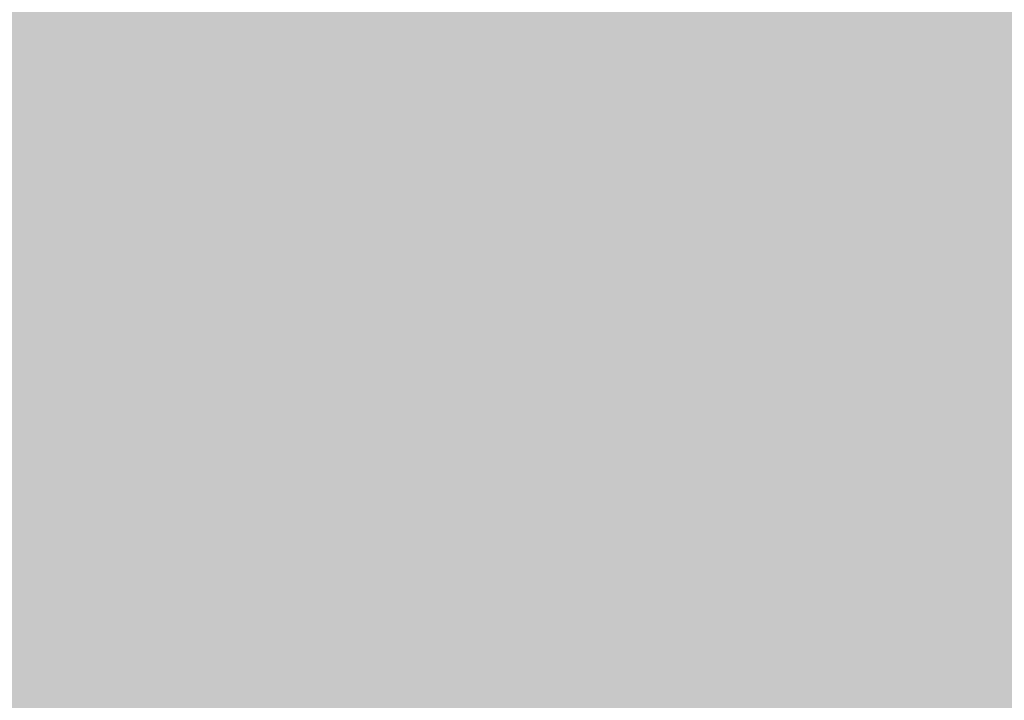
# Model space of a CAD drawing. Units: feet. Extents: x 3168 to 4724, y 827 to 1477.
# Tile 238 of 256: x 3382.8822 to 3383.8327, y 1098.344 to 1099.0007. Entities that reach past the tile are written whole.
import ezdxf

# ---------------------------------------------------------------- set-up
doc = ezdxf.new("R2010")
doc.units = ezdxf.units.FT
doc.layers.add('A-ELEV', color=7, linetype='Continuous', lineweight=35)
doc.layers.add('A-ELEV-PATT', color=8, linetype='Continuous', lineweight=13)

msp = doc.modelspace()

# ---------------------------------------------------------------- hatches: boundary and pattern name
at = {"layer": 'A-ELEV-PATT'}
h = msp.add_hatch(color=256, dxfattribs=at)
h.dxf.hatch_style = 1
edge = h.paths.add_edge_path()
edge.add_ellipse((3552.90576, 979.22014), major_axis=(36.74492, 0), ratio=0.48484848, start_angle=0, end_angle=360)
edge = h.paths.add_edge_path()
edge.add_ellipse((3559.89164, 929.25228), major_axis=(36.74492, 0), ratio=0.48484848, start_angle=0, end_angle=360)
edge = h.paths.add_edge_path()
edge.add_line((3299.31681, 1198.60608), (3479.91671, 1198.60608))
edge.add_line((3479.91671, 1198.60608), (3479.91671, 1209.86857))
edge.add_spline(control_points=[(3479.91671, 1209.86857), (3464.30116, 1209.86857), (3448.6856, 1209.86857), (3410.94914, 1209.86857), (3388.82823, 1209.86857), (3355.64688, 1209.86857), (3344.58642, 1209.86857), (3327.99574, 1209.86857), (3322.46552, 1209.86857), (3314.17018, 1209.86857), (3311.40507, 1209.86857), (3307.2574, 1209.86857), (3305.87484, 1209.86857), (3303.801, 1209.86857), (3303.10973, 1209.86857), (3302.07281, 1209.86857), (3301.72717, 1209.86857), (3301.20871, 1209.86857), (3301.03589, 1209.86857), (3300.77666, 1209.86857), (3300.69025, 1209.86857), (3300.56064, 1209.86857), (3300.51743, 1209.86857), (3300.45263, 1209.86857), (3300.43102, 1209.86857), (3300.39862, 1209.86857), (3300.38782, 1209.86857), (3300.36622, 1209.86857), (3300.34568, 1209.86857), (3300.34555, 1209.86857), (3300.3455, 1209.86857), (3300.3433, 1209.86857), (3300.34115, 1209.86857), (3300.33791, 1209.86857), (3300.33683, 1209.86857), (3300.33394, 1209.86857), (3300.33213, 1209.86857), (3300.32552, 1209.86858), (3300.32071, 1209.86858), (3300.31092, 1209.86859), (3300.30595, 1209.8686), (3300.29051, 1209.86862), (3300.28005, 1209.86865), (3300.23243, 1209.86878), (3300.1953, 1209.86895), (3299.95107, 1209.87061), (3299.74482, 1209.87433), (3299.43683, 1209.88326), (3299.33439, 1209.88679), (3299.18108, 1209.89292), (3299.13003, 1209.8951), (3298.65222, 1209.9168), (3298.22946, 1209.94572), (3297.60163, 1210.00237), (3297.3934, 1210.02346), (3297.08265, 1210.05831), (3296.97933, 1210.07046), (3296.29295, 1210.15486), (3295.71815, 1210.24336), (3294.86872, 1210.39885), (3294.5877, 1210.45448), (3294.16934, 1210.54335), (3294.03042, 1210.57388), (3291.70715, 1211.1012), (3289.65359, 1211.81344), (3285.77626, 1213.56399), (3283.95141, 1214.60348), (3280.51216, 1216.98008), (3278.89724, 1218.31759), (3276.37991, 1220.82949), (3275.41604, 1221.91774), (3274.03934, 1223.7077), (3273.58104, 1224.34953), (3273.14323, 1225.01632)], knot_values=[39.119033, 39.119033, 39.119033, 39.119033, 39.286353, 39.286353, 39.523379, 39.523379, 39.641892, 39.641892, 39.701148, 39.701148, 39.730777, 39.730777, 39.745591, 39.745591, 39.752998, 39.752998, 39.756701, 39.756701, 39.758553, 39.758553, 39.759479, 39.759479, 39.759942, 39.759942, 39.760173, 39.760173, 39.760289, 39.760289, 39.760405, 39.760405, 39.760463, 39.760463, 39.763389, 39.763389, 39.764851, 39.764851, 39.767304, 39.767304, 39.773825, 39.773825, 39.78057, 39.78057, 39.79477, 39.79477, 39.845194, 39.845194, 40.126715, 40.126715, 40.267476, 40.267476, 40.337856, 40.337856, 40.927023, 40.927023, 41.221606, 41.221606, 41.368898, 41.368898, 42.202622, 42.202622, 42.619485, 42.619485, 42.827916, 42.827916, 46.118323, 46.118323, 49.408731, 49.408731, 52.699139, 52.699139, 54.927489, 54.927489, 56.104228, 56.104228, 56.104228, 56.104228], weights=[1, 1, 1, 1, 1, 1, 1, 1, 1, 1, 1, 1, 1, 1, 1, 1, 1, 1, 1, 1, 1, 1, 1, 1, 1, 1, 1, 1, 1, 1, 1, 1, 1, 1, 1, 1, 1, 1, 1, 1, 1, 1, 1, 1, 1, 1, 1, 1, 1, 1, 1, 1, 1, 1, 1, 1, 1, 1, 1, 1, 1, 1, 1, 1, 1, 1, 1, 1, 1, 1, 1, 1, 1, 1], degree=3, periodic=0)
edge.add_line((3273.14323, 1225.01632), (3273.14323, 1099.01632))
edge.add_line((3273.14323, 1099.01632), (3299.31681, 1099.01632))
edge.add_line((3299.31681, 1099.01632), (3299.31681, 1198.60608))
edge = h.paths.add_edge_path()
edge.add_line((3304.75844, 1324.15806), (3479.91671, 1324.15806))
edge.add_line((3479.91671, 1324.15806), (3479.91671, 1335.71462))
edge.add_line((3479.91671, 1335.71462), (3269.16163, 1335.71462))
edge.add_spline(control_points=[(3269.16163, 1335.71462), (3264.02423, 1335.71462), (3258.36412, 1328.95819), (3259.26431, 1323.90027)], knot_values=[0, 0, 0, 0, 15.412191, 15.412191, 15.412191, 15.412191], degree=3, periodic=0)
edge.add_line((3259.26431, 1323.90027), (3265.51685, 1288.76913))
edge.add_line((3265.51685, 1288.76913), (3275.2651, 1261.54563))
edge.add_line((3275.2651, 1261.54563), (3304.75844, 1261.54563))
edge.add_line((3304.75844, 1261.54563), (3304.75844, 1324.15806))
h = msp.add_hatch(color=256, dxfattribs=at)
h.dxf.hatch_style = 1
h.paths.add_polyline_path([(3384.52525, 1099.01632), (3335.02917, 1099.01632), (3299.31681, 1099.01632), (3273.14323, 1099.01632), (3217.56536, 1099.01632), (3168.06928, 827.11626), (3335.02917, 827.11626)])

# ---------------------------------------------------------------- linework, layer by layer
at = {"layer": 'A-ELEV'}
msp.add_open_spline([(3808.5202, 1099.01632), (3808.5202, 1141.41324), (3808.5202, 1183.81015), (3808.5202, 1226.63532), (3808.5202, 1227.06358), (3808.5202, 1227.49183), (3811.49187, 1248.99467), (3814.46354, 1270.49752), (3817.46523, 1292.21756), (3817.49525, 1292.43476), (3817.52526, 1292.65196), (3817.5728, 1310.10675), (3817.62034, 1327.56153), (3817.66788, 1345.01632), (3817.66788, 1345.45796), (3817.66788, 1345.89961), (3817.66788, 1346.45605), (3817.66788, 1346.57084), (3817.66788, 1346.75289), (3817.66788, 1346.82014), (3817.66788, 1346.93487), (3817.66788, 1346.98234), (3817.66788, 1347.03859), (3817.66788, 1347.04736), (3817.66788, 1347.07366), (3817.66788, 1347.0593), (3817.66788, 1347.06155), (3817.66788, 1347.06267), (3817.66788, 1347.06603), (3817.66787, 1347.06827), (3817.66787, 1347.075), (3817.66787, 1347.07949), (3817.66785, 1347.09294), (3817.66783, 1347.1019), (3817.66777, 1347.12879), (3817.6677, 1347.1467), (3817.66743, 1347.20042), (3817.66716, 1347.23619), (3817.6661, 1347.34338), (3817.66504, 1347.41469), (3817.66081, 1347.62809), (3817.65661, 1347.76971), (3817.63997, 1348.19249), (3817.62351, 1348.47159), (3817.55909, 1349.30007), (3817.49612, 1349.84059), (3817.25543, 1351.42416), (3817.02632, 1352.42879), (3816.30687, 1354.88891), (3815.74375, 1356.26873), (3814.46396, 1358.81921), (3813.74641, 1359.99097), (3812.19584, 1362.17234), (3811.36225, 1363.18212), (3809.58884, 1365.06901), (3808.64882, 1365.94611), (3806.65426, 1367.57962), (3805.5997, 1368.33615), (3803.35289, 1369.72233), (3802.16054, 1370.35239), (3799.60081, 1371.45359), (3798.23269, 1371.92548), (3795.28008, 1372.63462), (3793.69315, 1372.87207), (3791.86944, 1372.92648), (3791.74086, 1372.92922), (3791.35337, 1372.9341), (3791.09271, 1372.9329), (3790.30412, 1372.91507), (3789.76954, 1372.88419), (3789.20919, 1372.83024), (3789.19062, 1372.82842), (3789.13489, 1372.82291), (3789.0977, 1372.81914), (3789.04844, 1372.81401), (3789.0364, 1372.81274), (3789.00026, 1372.80892), (3788.97615, 1372.80633), (3788.9494, 1372.8034), (3788.94679, 1372.80312), (3788.94257, 1372.80266), (3788.94097, 1372.80248), (3788.93857, 1372.80222), (3788.93778, 1372.80213), (3788.93539, 1372.80187), (3788.86753, 1372.7944), (3788.75687, 1372.78223), (3788.70153, 1372.77614), (3788.53553, 1372.75788), (3788.42486, 1372.74571), (3788.09286, 1372.70918), (3787.87152, 1372.68484), (3787.20751, 1372.61179), (3786.76483, 1372.5631), (3785.43681, 1372.41701), (3784.55147, 1372.31962), (3781.89542, 1372.02744), (3780.12473, 1371.83266), (3774.81265, 1371.24831), (3771.27126, 1370.85874), (3760.64709, 1369.69004), (3753.56431, 1368.9109), (3732.31597, 1366.5735), (3718.15042, 1365.01523), (3694.00676, 1362.35933), (3684.02866, 1361.26169), (3674.05056, 1360.16406), (3664.60066, 1360.16406), (3655.15077, 1360.16406), (3626.80108, 1360.16406), (3607.90129, 1360.16406), (3551.20192, 1360.16406), (3513.40234, 1360.16406), (3467.72518, 1360.16406), (3459.8476, 1360.16406), (3436.21487, 1360.16406), (3420.45972, 1360.16406), (3373.19425, 1360.16406), (3341.68395, 1360.16406), (3302.84816, 1360.16406), (3295.52269, 1360.16406), (3286.03829, 1360.16406), (3283.87937, 1360.16406), (3277.40261, 1360.16406), (3273.08477, 1360.16406), (3267.73285, 1360.16406), (3266.69877, 1360.16406), (3263.59652, 1360.16406), (3261.52835, 1360.16406), (3259.23694, 1360.16406), (3259.0137, 1360.16406), (3258.34396, 1360.16406), (3257.89747, 1360.16406), (3257.431, 1360.16406), (3257.41102, 1360.16406), (3257.37057, 1360.16406), (3257.37547, 1360.16406), (3257.3746, 1360.16406), (3257.37394, 1360.16406), (3257.37196, 1360.16406), (3257.37064, 1360.16406), (3257.36667, 1360.16406), (3257.36403, 1360.16406), (3257.35611, 1360.16405), (3257.35083, 1360.16405), (3257.33499, 1360.16402), (3257.32443, 1360.164), (3257.29277, 1360.1639), (3257.27168, 1360.1638), (3257.20844, 1360.1634), (3257.16634, 1360.163), (3257.04021, 1360.16139), (3256.95635, 1360.15978), (3256.7055, 1360.15339), (3256.53924, 1360.14704), (3256.04357, 1360.12192), (3255.7173, 1360.0971), (3254.75245, 1360.00048), (3254.12797, 1359.90651), (3252.18007, 1359.52533), (3250.94157, 1359.14399), (3248.67018, 1358.24329), (3247.63574, 1357.72383), (3245.73263, 1356.60347), (3244.86339, 1356.00206), (3243.25311, 1354.74287), (3242.51197, 1354.08473), (3240.75105, 1352.34478), (3239.80096, 1351.22957), (3238.08777, 1348.87244), (3237.32469, 1347.63036), (3235.98251, 1344.97163), (3235.40221, 1343.55491), (3234.59108, 1340.81546), (3234.31088, 1339.54355), (3233.97649, 1336.80256), (3233.92211, 1335.33088), (3234.14892, 1332.59127), (3234.34953, 1331.3672), (3234.71989, 1329.99937), (3234.75242, 1329.88336), (3234.85362, 1329.5348), (3234.92589, 1329.30168), (3235.02484, 1329.00255), (3235.04692, 1328.93693), (3235.07764, 1328.84724), (3235.08592, 1328.8232), (3235.11094, 1328.75106), (3235.12783, 1328.70296), (3235.14799, 1328.64624), (3235.15106, 1328.63763), (3235.1561, 1328.62353), (3235.15806, 1328.61803), (3235.16021, 1328.61203), (3235.16561, 1328.59694), (3235.1801, 1328.55649), (3235.19026, 1328.5281), (3235.22076, 1328.44295), (3235.24108, 1328.38618), (3235.30207, 1328.21587), (3235.34273, 1328.10232), (3235.4647, 1327.7617), (3235.54601, 1327.53462), (3235.78995, 1326.85338), (3235.95258, 1326.39922), (3236.44046, 1325.03674), (3236.76571, 1324.12841), (3237.74148, 1321.40345), (3238.39198, 1319.5868), (3240.34351, 1314.13687), (3241.64452, 1310.50358), (3245.54757, 1299.60371), (3248.14961, 1292.33713), (3255.95571, 1270.53739), (3261.15977, 1256.00423), (3267.38762, 1238.612), (3268.4114, 1235.75294), (3269.51038, 1232.68386), (3269.58558, 1232.47385), (3269.70661, 1232.13585), (3269.75244, 1232.00786), (3269.82733, 1231.79873), (3269.85638, 1231.7176), (3269.90632, 1231.57812), (3269.92721, 1231.51978), (3269.97247, 1231.39341), (3269.99683, 1231.32537), (3270.0265, 1231.24251), (3270.03181, 1231.22768), (3270.04028, 1231.20402), (3270.03922, 1231.20698), (3270.03936, 1231.2066), (3270.03943, 1231.20641), (3270.03963, 1231.20585), (3270.03977, 1231.20547), (3270.04017, 1231.20433), (3270.04044, 1231.20358), (3270.04125, 1231.20131), (3270.0418, 1231.1998), (3270.04342, 1231.19527), (3270.0445, 1231.19225), (3270.04776, 1231.18318), (3270.04993, 1231.17714), (3270.05644, 1231.15903), (3270.06079, 1231.14696), (3270.07387, 1231.11076), (3270.08261, 1231.08666), (3270.10894, 1231.01441), (3270.1266, 1230.96635), (3270.17993, 1230.82246), (3270.21595, 1230.72692), (3270.32532, 1230.44151), (3270.40003, 1230.25281), (3270.62925, 1229.69144), (3270.78888, 1229.3235), (3271.28649, 1228.23832), (3271.6431, 1227.53975), (3272.77586, 1225.51528), (3273.61417, 1224.2605), (3275.41604, 1221.91774), (3276.37991, 1220.82949), (3278.89724, 1218.31759), (3280.51216, 1216.98008), (3283.95141, 1214.60348), (3285.77626, 1213.56399), (3289.65359, 1211.81344), (3291.70715, 1211.1012), (3294.03042, 1210.57388), (3294.16934, 1210.54335), (3294.5877, 1210.45448), (3294.86872, 1210.39885), (3295.71815, 1210.24336), (3296.29295, 1210.15486), (3296.97933, 1210.07046), (3297.08265, 1210.05831), (3297.3934, 1210.02346), (3297.60163, 1210.00237), (3298.22946, 1209.94572), (3298.65222, 1209.9168), (3299.13003, 1209.8951), (3299.18108, 1209.89292), (3299.33439, 1209.88679), (3299.43683, 1209.88326), (3299.74482, 1209.87433), (3299.95107, 1209.87061), (3300.1953, 1209.86895), (3300.23243, 1209.86878), (3300.28005, 1209.86865), (3300.29051, 1209.86862), (3300.30595, 1209.8686), (3300.31092, 1209.86859), (3300.32071, 1209.86858), (3300.32552, 1209.86858), (3300.33213, 1209.86857), (3300.33394, 1209.86857), (3300.33683, 1209.86857), (3300.33791, 1209.86857), (3300.34115, 1209.86857), (3300.3433, 1209.86857), (3300.3455, 1209.86857), (3300.34555, 1209.86857), (3300.34568, 1209.86857), (3300.36622, 1209.86857), (3300.38782, 1209.86857), (3300.39862, 1209.86857), (3300.43102, 1209.86857), (3300.45263, 1209.86857), (3300.51743, 1209.86857), (3300.56064, 1209.86857), (3300.69025, 1209.86857), (3300.77666, 1209.86857), (3301.03589, 1209.86857), (3301.20871, 1209.86857), (3301.72717, 1209.86857), (3302.07281, 1209.86857), (3303.10973, 1209.86857), (3303.801, 1209.86857), (3305.87484, 1209.86857), (3307.2574, 1209.86857), (3311.40507, 1209.86857), (3314.17018, 1209.86857), (3322.46552, 1209.86857), (3327.99574, 1209.86857), (3344.58642, 1209.86857), (3355.64688, 1209.86857), (3388.82823, 1209.86857), (3410.94914, 1209.86857), (3477.31185, 1209.86857), (3521.55366, 1209.86857), (3566.83618, 1209.86857), (3567.87689, 1209.86857), (3570.99902, 1209.86857), (3573.08043, 1209.86857), (3575.7814, 1209.86857), (3576.40094, 1209.86857), (3577.29582, 1209.86857), (3577.57115, 1209.86857), (3578.39715, 1209.86857), (3578.94781, 1209.86857), (3579.75649, 1209.86857), (3580.01451, 1209.86857), (3580.34274, 1209.86857), (3580.32686, 1209.86857), (3580.32717, 1209.86857), (3580.32732, 1209.86857), (3580.32778, 1209.86857), (3580.32809, 1209.86857), (3580.329, 1209.86857), (3580.32961, 1209.86857), (3580.33145, 1209.86857), (3580.33267, 1209.86857), (3580.33633, 1209.86857), (3580.33878, 1209.86857), (3580.34611, 1209.86856), (3580.35099, 1209.86856), (3580.36566, 1209.86854), (3580.37544, 1209.86852), (3580.4048, 1209.86845), (3580.42439, 1209.86838), (3580.48318, 1209.86808), (3580.52244, 1209.86779), (3580.64036, 1209.86662), (3580.71919, 1209.86545), (3580.95632, 1209.86077), (3581.11522, 1209.85607), (3581.59416, 1209.83723), (3581.91642, 1209.81833), (3582.88995, 1209.74243), (3583.54799, 1209.66617), (3585.53183, 1209.36062), (3586.86722, 1209.05389), (3589.47155, 1208.25247), (3590.74024, 1207.75785), (3591.99545, 1207.1588), (3592.05781, 1207.12874), (3592.24424, 1207.03795), (3592.36768, 1206.97663), (3592.73528, 1206.79036), (3592.97675, 1206.6631), (3593.24454, 1206.51644), (3593.27473, 1206.49982), (3593.36512, 1206.44984), (3593.42511, 1206.41633), (3593.60431, 1206.31529), (3593.72273, 1206.24721), (3593.85721, 1206.1684), (3593.87436, 1206.15832), (3593.92574, 1206.12804), (3593.9599, 1206.1078), (3594.06209, 1206.0469), (3594.12983, 1206.00607), (3594.20844, 1205.95817), (3594.21968, 1205.9513), (3594.25339, 1205.93069), (3594.27582, 1205.91692), (3594.34297, 1205.87554), (3594.38756, 1205.84785), (3594.43362, 1205.81905), (3594.43526, 1205.81802), (3594.44017, 1205.81495), (3594.44345, 1205.81289), (3594.44712, 1205.81059), (3594.44752, 1205.81035), (3594.44869, 1205.80961), (3594.44948, 1205.80912), (3594.45037, 1205.80856), (3594.45047, 1205.8085), (3594.4506, 1205.80842), (3594.4674, 1205.79789), (3594.49327, 1205.78167), (3594.5062, 1205.77357), (3594.54501, 1205.74925), (3594.57088, 1205.73303), (3594.64849, 1205.6844), (3594.70023, 1205.65197), (3594.85544, 1205.55469), (3594.95892, 1205.48984), (3595.26936, 1205.29528), (3595.47631, 1205.16558), (3596.09719, 1204.77646), (3596.5111, 1204.51705), (3597.75284, 1203.73883), (3598.58067, 1203.22001), (3601.06415, 1201.66355), (3602.71981, 1200.62591), (3607.68677, 1197.513), (3610.99809, 1195.43773), (3620.93202, 1189.2119), (3627.55464, 1185.06135), (3647.42251, 1172.60971), (3660.66775, 1164.30861), (3700.40348, 1139.40531), (3726.89397, 1122.80312), (3757.20572, 1103.80605), (3761.02697, 1101.41118), (3764.84822, 1099.01632), (3745.32827, 1099.01632), (3725.80832, 1099.01632), (3706.28837, 1099.01632), (3706.28837, 1108.45324), (3706.28837, 1117.89016), (3706.28837, 1127.32708), (3710.75075, 1127.32708), (3715.21314, 1127.32708), (3719.67553, 1127.32708)], degree=3, knots=[0, 0, 0, 0, 0.982037, 0.982037, 0.991957, 0.991957, 0.991957, 1.966522, 1.966522, 1.976367, 1.976367, 1.976367, 2.976367, 2.976367, 2.976367, 3.00169, 3.00169, 3.008272, 3.008272, 3.012129, 3.012129, 3.014851, 3.014851, 3.015353, 3.015353, 3.016359, 3.016359, 3.017365, 3.017365, 3.019376, 3.019376, 3.023398, 3.023398, 3.031442, 3.031442, 3.047531, 3.047531, 3.079708, 3.079708, 3.144063, 3.144063, 3.272772, 3.272772, 3.53019, 3.53019, 4.045026, 4.045026, 5.074698, 5.074698, 6.700878, 6.700878, 8.327058, 8.327058, 9.953238, 9.953238, 11.579418, 11.579418, 13.205598, 13.205598, 14.831778, 14.831778, 16.457958, 16.457958, 18.084138, 18.084138, 18.206872, 18.206872, 18.45234, 18.45234, 18.943275, 18.943275, 18.960093, 18.960093, 18.993729, 18.993729, 19.00461, 19.00461, 19.026374, 19.026374, 19.028737, 19.028737, 19.03018, 19.03018, 19.030897, 19.030897, 19.032332, 19.032332, 19.033766, 19.033766, 19.036636, 19.036636, 19.042374, 19.042374, 19.053851, 19.053851, 19.076805, 19.076805, 19.122714, 19.122714, 19.21453, 19.21453, 19.398163, 19.398163, 19.765429, 19.765429, 20.024128, 20.024128, 20.024128, 20.092031, 20.092031, 20.227836, 20.227836, 20.499446, 20.499446, 20.556051, 20.556051, 20.66926, 20.66926, 20.895678, 20.895678, 20.948316, 20.948316, 20.963829, 20.963829, 20.994855, 20.994855, 21.002285, 21.002285, 21.017146, 21.017146, 21.01875, 21.01875, 21.021959, 21.021959, 21.022102, 21.022102, 21.022249, 21.022249, 21.022708, 21.022708, 21.023627, 21.023627, 21.025464, 21.025464, 21.029138, 21.029138, 21.036486, 21.036486, 21.051183, 21.051183, 21.080575, 21.080575, 21.139361, 21.139361, 21.256932, 21.256932, 21.492073, 21.492073, 21.962356, 21.962356, 23.01002, 23.01002, 24.057684, 24.057684, 25.105348, 25.105348, 26.153011, 26.153011, 27.776787, 27.776787, 29.400562, 29.400562, 31.024337, 31.024337, 32.278801, 32.278801, 33.533265, 33.533265, 34.467568, 34.467568, 34.553971, 34.553971, 34.726776, 34.726776, 34.775309, 34.775309, 34.793079, 34.793079, 34.82862, 34.82862, 34.834979, 34.834979, 34.839039, 34.839039, 34.839411, 34.839411, 34.840285, 34.840285, 34.842034, 34.842034, 34.845531, 34.845531, 34.852525, 34.852525, 34.866512, 34.866512, 34.894488, 34.894488, 34.950439, 34.950439, 35.062342, 35.062342, 35.286147, 35.286147, 35.733758, 35.733758, 35.821815, 35.821815, 35.828283, 35.828283, 35.832225, 35.832225, 35.834724, 35.834724, 35.836521, 35.836521, 35.838617, 35.838617, 35.839073, 35.839073, 35.839345, 35.839345, 35.839617, 35.839617, 35.840161, 35.840161, 35.841249, 35.841249, 35.843425, 35.843425, 35.847778, 35.847778, 35.856482, 35.856482, 35.873891, 35.873891, 35.908709, 35.908709, 35.978345, 35.978345, 36.117617, 36.117617, 36.396161, 36.396161, 36.953248, 36.953248, 38.067423, 38.067423, 40.295772, 40.295772, 42.524122, 42.524122, 45.81453, 45.81453, 49.104937, 49.104937, 52.395345, 52.395345, 52.603776, 52.603776, 53.020639, 53.020639, 53.854363, 53.854363, 54.001655, 54.001655, 54.296238, 54.296238, 54.885405, 54.885405, 54.955785, 54.955785, 55.096546, 55.096546, 55.378067, 55.378067, 55.42849, 55.42849, 55.442691, 55.442691, 55.449436, 55.449436, 55.455957, 55.455957, 55.458409, 55.458409, 55.459872, 55.459872, 55.462798, 55.462798, 55.462856, 55.462856, 55.462972, 55.462972, 55.463088, 55.463088, 55.463319, 55.463319, 55.463782, 55.463782, 55.464708, 55.464708, 55.46656, 55.46656, 55.470263, 55.470263, 55.47767, 55.47767, 55.492484, 55.492484, 55.522112, 55.522112, 55.581369, 55.581369, 55.699882, 55.699882, 55.936907, 55.936907, 56.410959, 56.410959, 56.42211, 56.42211, 56.444413, 56.444413, 56.451051, 56.451051, 56.454001, 56.454001, 56.459901, 56.459901, 56.462666, 56.462666, 56.463418, 56.463418, 56.464171, 56.464171, 56.465675, 56.465675, 56.468684, 56.468684, 56.474702, 56.474702, 56.486738, 56.486738, 56.51081, 56.51081, 56.558955, 56.558955, 56.655243, 56.655243, 56.847821, 56.847821, 57.232975, 57.232975, 58.003284, 58.003284, 59.543901, 59.543901, 62.625137, 62.625137, 68.787607, 68.787607, 74.950078, 74.950078, 75.27336, 75.27336, 75.919923, 75.919923, 77.213051, 77.213051, 77.377769, 77.377769, 77.707206, 77.707206, 78.366079, 78.366079, 78.462532, 78.462532, 78.655436, 78.655436, 79.041245, 79.041245, 79.105735, 79.105735, 79.234714, 79.234714, 79.492672, 79.492672, 79.502197, 79.502197, 79.521249, 79.521249, 79.523534, 79.523534, 79.528103, 79.528103, 79.528682, 79.528682, 79.528885, 79.528885, 79.529089, 79.529089, 79.529495, 79.529495, 79.530308, 79.530308, 79.531935, 79.531935, 79.535187, 79.535187, 79.541693, 79.541693, 79.554704, 79.554704, 79.580725, 79.580725, 79.632769, 79.632769, 79.736856, 79.736856, 79.94503, 79.94503, 80.361377, 80.361377, 80.421435, 80.421435, 80.421435, 81.421435, 81.421435, 81.421435, 82.421435, 82.421435, 82.421435, 83.421435, 83.421435, 83.421435, 83.421435], dxfattribs=at)

doc.saveas('drawing.dxf')
